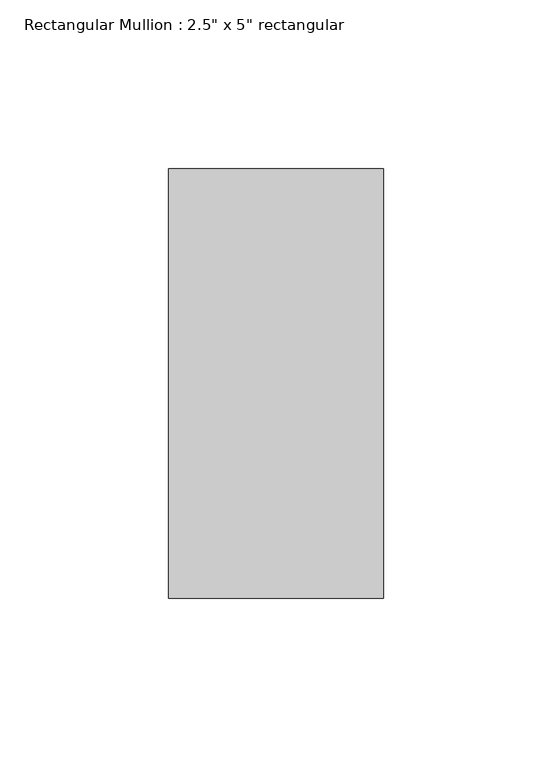
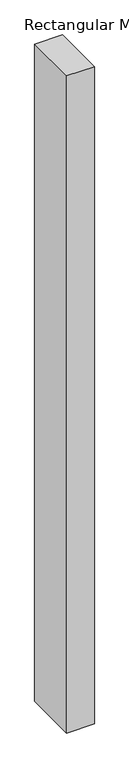
"""IFC4 building model written with IfcOpenShell, lengths in millimetres: member geometry."""

from ifc_helpers import new_model, si_unit, frame, origin, place, context, project, spatial, polyline, outline, extrude, source, transform, mapped, element, save


def member_ea832cfd(model_context):
    return source(origin(), model_context, "Body", "SweptSolid", [
        extrude(outline(polyline([(31.75, 63.5), (31.75, -63.5), (-31.75, -63.5), (-31.75, 63.5), (31.75, 63.5)])), frame((0.0, 0.0, -1593.2699234), z_axis=(0.0, 0.0, 1.0), x_axis=(1.0, 0.0, 0.0)), (0.0, 0.0, 1.0), 1593.2699234),
    ])


if __name__ == "__main__":
    model = new_model("IFC4")
    model_context = context("Model", 3, world=origin())
    ifc_project = project(units=[si_unit("LENGTHUNIT", "METRE", prefix="MILLI")], contexts=[model_context])
    site = spatial("IfcSite", under=ifc_project)
    building = spatial("IfcBuilding", under=site)
    placement = place(None, origin())
    member_shape = member_ea832cfd(model_context)
    element("IfcMember", 1, ObjectType="Rectangular Mullion : 2.5\" x 5\" rectangular", at=placement, inside=building, context=model_context, shape_type="MappedRepresentation", body=[
        mapped(member_shape, transform((0.0, 0.0, 0.0), x_axis=(1.0, 0.0, 0.0), y_axis=(0.0, 1.0, 0.0), z_axis=(0.0, 0.0, 1.0))),
    ])
    save(model, "model.ifc")

# Revit data of these elements
# Type "Rectangular Mullion : 2.5\" x 5\" rectangular"
#   built-in parameter 1007304 = 0.416667 (stored number, unit not read)
#   built-in parameter 1007301 = 0.104167 (stored number, unit not read)
#   built-in parameter 1007300 = 0.104167 (stored number, unit not read)
# Element 1 (IfcMember, "Rectangular Mullion : 2.5\" x 5\" rectangular")
#   Materials on its faces: "Aluminum"
# Materials
#   "Aluminum": class "Metal", colour RGB 247 247 247, transparency 0, Description = "Aluminum 6061", Cost = 0
